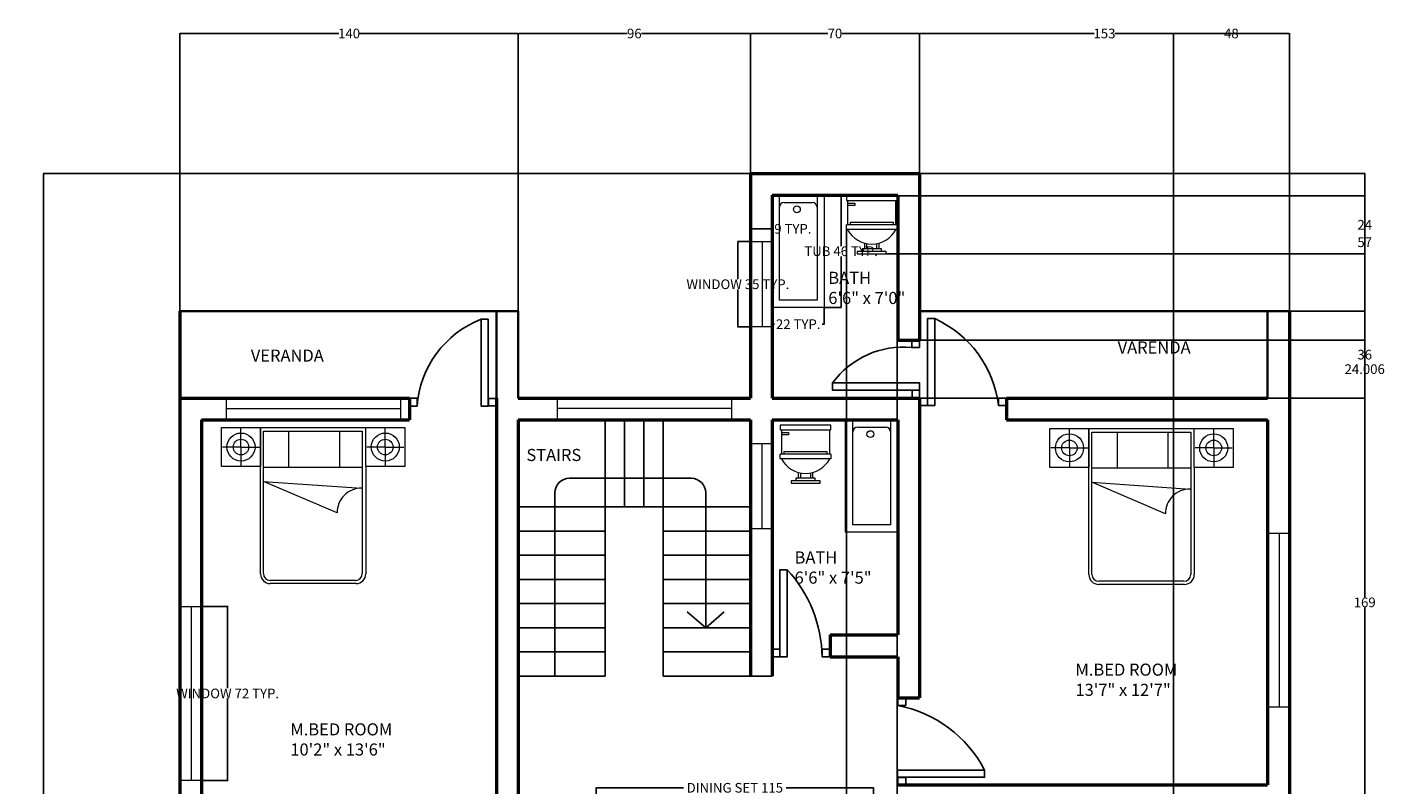
# Model space of a CAD drawing. Units: inches. Extents: x 870 to 1431, y 383 to 1070.
# Tile 9 of 9: x 870 to 1431, y 756 to 1070. Entities that reach past the tile are written whole.
import ezdxf

# ---------------------------------------------------------------- set-up
doc = ezdxf.new("R2010")
doc.units = ezdxf.units.IN
doc.header["$MEASUREMENT"] = 0
for name, color, linetype, lineweight in [('A-ANNO-DIMS', 2, 'Continuous', 18), ('A-AREA-IDEN', 7, 'Continuous', 25), ('A-DOOR', 3, 'Continuous', 25), ('A-FLOR-EXTR', 7, 'Continuous', 35), ('A-FLOR-FIXT', 9, 'Continuous', 18), ('A-FLOR-STRS', 7, 'Continuous', 25), ('A-FURN', 8, 'Continuous', 18), ('A-GLAZ', 4, 'Continuous', 18), ('A-WALL', 7, 'Continuous', 50)]:
    doc.layers.add(name, color=color, linetype=linetype, lineweight=lineweight)
doc.styles.get("Standard").update_dxf_attribs({"font": 'arial.ttf'})
doc.dimstyles.get("Standard").update_dxf_attribs({"dimtxt": 4, "dimasz": 0.18, "dimexe": 0.18, "dimexo": 0.0625, "dimgap": 0.09, "dimtad": 0, "dimtih": 1, "dimtoh": 1, "dimdec": 0, "dimrnd": 6, "dimzin": 0, "dimdsep": 46, "dimlunit": 3, "dimtxsty": 'Standard', "dimcen": 0.09, "dimadec": 0, "dimazin": 0, "dimtfac": 1, "dimtdec": 0, "dimtofl": 0, "dimtmove": 0, "dimatfit": 3, "dimfxl": 1, "dimtolj": 1, "dimtzin": 0, "dimarcsym": 0})

# ---------------------------------------------------------------- blocks, each defined once
blk = doc.blocks.new('A$C65997121')
for p, q in [((0, 1.5, -0.169), (0, 2, -0.169)), ((0, 2, -0.169), (0.5, 2, -0.169)), ((0, 1.5, -0.169), (0, 2, -0.169)), ((0, 2, -0.169), (0.5, 2, -0.169)), ((0.25, 1.75, -0.169), (0.25, 1.988, -0.169)), ((0.5, 2, -0.169), (1.755, 2, -0.169)), ((0.5, 2, -0.169), (1.512, 2, -0.169)), ((0.5, 2, -0.169), (1.512, 2, -0.169)), ((0.5, 0.125, -0.169), (0.5, 2, -0.169)), ((0.5, 2, -0.169), (0.5, 1.5, -0.169)), ((0.538, 1.488, -0.169), (0.538, 1.952, -0.169)), ((0.538, 1.952, -0.169), (1.805, 1.952, -0.169)), ((0.86, 1.952, -0.169), (0.86, 1.488, -0.169)), ((1.512, 2, -0.169), (2.35, 2, -0.169)), ((1.512, 2, -0.169), (2.35, 2, -0.169)), ((1.512, 1.952, -0.169), (1.512, 1.488, -0.169)), ((1.805, 1.952, -0.169), (1.805, 1.488, -0.169)), ((1.85, 2, -0.169), (2.35, 2, -0.169)), ((1.85, 1.5, -0.169), (1.85, 2, -0.169)), ((2.1, 1.75, -0.169), (2.1, 1.988, -0.169)), ((2.35, 2, -0.169), (2.35, 1.5, -0.169)), ((2.35, 2, -0.169), (2.35, 1.5, -0.169)), ((2.35, 2, -0.169), (2.35, 1.5, -0.169)), ((0.25, 1.75, -0.169), (0.012, 1.75, -0.169)), ((0.25, 1.75, -0.169), (0.25, 1.512, -0.169)), ((0.25, 1.75, -0.169), (0.488, 1.75, -0.169)), ((2.1, 1.75, -0.169), (1.862, 1.75, -0.169)), ((2.1, 1.75, -0.169), (2.338, 1.75, -0.169)), ((2.1, 1.75, -0.169), (2.1, 1.512, -0.169)), ((0.5, 1.5, -0.169), (0, 1.5, -0.169)), ((0.5, 1.5, -0.169), (0, 1.5, -0.169)), ((0.5, 0.125, -0.169), (0.5, 1.5, -0.169)), ((1.805, 1.488, -0.169), (0.538, 1.488, -0.169)), ((0.538, 0.128, -0.169), (0.538, 1.488, -0.169)), ((1.805, 1.488, -0.169), (1.805, 0.128, -0.169)), ((2.35, 1.5, -0.169), (1.85, 1.5, -0.169)), ((2.35, 1.5, -0.169), (1.85, 1.5, -0.169)), ((1.85, 1.5, -0.169), (1.85, 0.125, -0.169)), ((2.35, 1.5, -0.169), (1.85, 1.5, -0.169)), ((1.85, 1.5, -0.169), (1.85, 0.125, -0.169)), ((1.483, 0.905, -0.506), (0.538, 1.31, -0.506)), ((0.538, 1.31, -0.506), (1.797, 1.222, -0.506)), ((1.717, 0.04, -0.169), (0.625, 0.04, -0.169)), ((1.725, 0, -0.169), (0.625, 0, -0.169)), ((1.725, 0, -0.169), (0.625, 0, -0.169))]:
    blk.add_line(p, q)
for centre, radius in [((0.25, 1.75, -0.169), 0.18), ((2.1, 1.75, -0.169), 0.18), ((0.25, 1.75, -0.169), 0.1), ((2.1, 1.75, -0.169), 0.1)]:
    blk.add_circle(centre, radius)
for centre, radius, start, end in [((1.793, 0.911, -0.506), 0.311, 89.3268, 181.1229), ((0.625, 0.125, -0.169), 0.125, 179.9939, 269.9939), ((0.625, 0.125, -0.169), 0.125, 179.9939, 269.9939), ((0.625, 0.128, -0.169), 0.0875, 179.9939, 269.9939), ((1.717, 0.128, -0.169), 0.0875, 269.9939, 359.9939), ((1.725, 0.125, -0.169), 0.125, 269.9939, 359.9939), ((1.725, 0.125, -0.169), 0.125, 269.9939, 359.9939)]:
    blk.add_arc(centre, radius, start, end)
blk = doc.blocks.new('Toilet - Imperial')
for p, q in [((-10, 22), (-10, 12)), ((-10, 21), (-7, 21)), ((-7, 20), (-10, 20)), ((-7, 21), (-7, 20)), ((10, 12), (10, 22)), ((10.5, 12), (-10.5, 12)), ((-10.5, 10), (-10.5, 12)), ((9, 13), (-9, 13)), ((-9, 13), (-9, 12)), ((9, 12), (9, 13)), ((10.5, 12), (10.5, 10)), ((10.5, 10), (-10.5, 10)), ((4, 2), (-4, 2)), ((-4, 2), (-4, 1)), ((-3, 4.4065), (-3, 2)), ((-2, 2), (-2, 4.1658)), ((2, 4.1658), (2, 2)), ((3, 2), (3, 4.4065)), ((4, 1), (4, 2))]:
    blk.add_line(p, q)
for points in [[(10.5, 22), (10.5, 24), (-10.5, 24), (-10.5, 22)], [(6, 0), (6, 1), (-6, 1), (-6, 0)]]:
    blk.add_lwpolyline(points, close=True)
blk.add_arc((0, 15.3333), 11.3333, 208.0725, 331.9275)
blk = doc.blocks.new('WIN-72IN')
blk.add_line((4.72, 72), (4.72, 0))
blk.add_lwpolyline([(0, 72), (9, 72), (9, 0), (0, 0)], close=True)
blk = doc.blocks.new('WIN-BATH-35IN')
blk.add_line((4.73, 35.25), (4.73, 0))
blk.add_lwpolyline([(0, 0), (0, 35.25), (9, 35.25), (9, 0)], close=True)
blk = doc.blocks.new('BATH-TUB-COMPACT')
for p, q in [((0, 46.44), (21.59, 46.44)), ((0, 0), (0, 46.44)), ((3, 3), (3, 46.44)), ((18.59, 46.44), (18.59, 3)), ((21.59, 46.44), (21.59, 0)), ((5, 43.44), (16.59, 43.44)), ((21.59, 0), (0, 0)), ((18.59, 3), (3, 3))]:
    blk.add_line(p, q)
blk.add_circle((10.26, 40.55), 1.41)
for centre, start, end in [((5, 41.44), 90, 180), ((16.59, 41.44), 0, 90)]:
    blk.add_arc(centre, 2, start, end)
blk = doc.blocks.new('*D105')
at = {"layer": 'A-ANNO-DIMS', "color": 0, "lineweight": -2, "transparency": 16777216}
for p, q in [((941.8, 830.29), (952.72, 830.29)), ((952.54, 830.11), (952.54, 796.45)), ((952.54, 758.47), (952.54, 792.14)), ((941.8, 758.29), (952.72, 758.29))]:
    blk.add_line(p, q, dxfattribs=at)
at = {"layer": 'A-ANNO-DIMS', "color": 0, "transparency": 16777216}
for points in [[(952.51, 830.11), (952.57, 830.11), (952.54, 830.29)], [(952.51, 758.47), (952.57, 758.47), (952.54, 758.29)]]:
    blk.add_solid(points, dxfattribs=at)
at = {"layer": 'Defpoints', "color": 0, "transparency": 16777216}
for p in [(941.74, 830.29), (952.54, 830.29), (941.74, 758.29)]:
    blk.add_point(p, dxfattribs=at)
at = {"layer": 'A-ANNO-DIMS', "color": 0, "transparency": 16777216, "insert": (952.54, 794.29), "char_height": 4, "attachment_point": 5}
blk.add_mtext('\\A1;WINDOW 72 TYP.', dxfattribs=at)
blk = doc.blocks.new('*D106')
at = {"layer": 'A-ANNO-DIMS', "color": 0, "lineweight": -2, "transparency": 16777216}
for p, q in [((932.74, 758.23), (932.74, 747.31)), ((941.74, 758.23), (941.74, 747.31)), ((932.92, 747.49), (941.56, 747.49)), ((941.74, 747.49), (941.92, 747.49))]:
    blk.add_line(p, q, dxfattribs=at)
at = {"layer": 'A-ANNO-DIMS', "color": 0, "transparency": 16777216}
for points in [[(932.92, 747.52), (932.92, 747.46), (932.74, 747.49)], [(941.56, 747.52), (941.56, 747.46), (941.74, 747.49)]]:
    blk.add_solid(points, dxfattribs=at)
at = {"layer": 'Defpoints', "color": 0, "transparency": 16777216}
for p in [(932.74, 758.29), (941.74, 758.29), (941.74, 747.49)]:
    blk.add_point(p, dxfattribs=at)
at = {"layer": 'A-ANNO-DIMS', "color": 0, "transparency": 16777216, "insert": (950.19, 747.49), "char_height": 4, "attachment_point": 5}
blk.add_mtext('\\A1;9 TYP.', dxfattribs=at)
blk = doc.blocks.new('*D111')
at = {"layer": 'A-ANNO-DIMS', "color": 0, "lineweight": -2, "transparency": 16777216}
for p, q in [((1168.86, 981.23), (1163.46, 981.23)), ((1163.64, 981.05), (1163.64, 965.76)), ((1163.64, 946.16), (1163.64, 961.44)), ((1168.86, 945.98), (1163.46, 945.98))]:
    blk.add_line(p, q, dxfattribs=at)
at = {"layer": 'A-ANNO-DIMS', "color": 0, "transparency": 16777216}
for points in [[(1163.61, 981.05), (1163.67, 981.05), (1163.64, 981.23)], [(1163.61, 946.16), (1163.67, 946.16), (1163.64, 945.98)]]:
    blk.add_solid(points, dxfattribs=at)
at = {"layer": 'Defpoints', "color": 0, "transparency": 16777216}
for p in [(1163.64, 981.23), (1168.93, 981.23), (1168.93, 945.98)]:
    blk.add_point(p, dxfattribs=at)
at = {"layer": 'A-ANNO-DIMS', "color": 0, "transparency": 16777216, "insert": (1163.64, 963.6), "char_height": 4, "attachment_point": 5}
blk.add_mtext('\\A1;WINDOW 35 TYP.', dxfattribs=at)
blk = doc.blocks.new('*D112')
at = {"layer": 'A-ANNO-DIMS', "color": 0, "lineweight": -2, "transparency": 16777216}
for p, q in [((1168.93, 981.29), (1168.93, 986.7)), ((1169.11, 986.52), (1177.75, 986.52)), ((1177.93, 981.29), (1177.93, 986.7)), ((1177.93, 986.52), (1178.11, 986.52))]:
    blk.add_line(p, q, dxfattribs=at)
at = {"layer": 'A-ANNO-DIMS', "color": 0, "transparency": 16777216}
for points in [[(1169.11, 986.55), (1169.11, 986.49), (1168.93, 986.52)], [(1177.75, 986.55), (1177.75, 986.49), (1177.93, 986.52)]]:
    blk.add_solid(points, dxfattribs=at)
at = {"layer": 'Defpoints', "color": 0, "transparency": 16777216}
for p in [(1177.93, 986.52), (1168.93, 981.23), (1177.93, 981.23)]:
    blk.add_point(p, dxfattribs=at)
at = {"layer": 'A-ANNO-DIMS', "color": 0, "transparency": 16777216, "insert": (1186.38, 986.52), "char_height": 4, "attachment_point": 5}
blk.add_mtext('\\A1;9 TYP.', dxfattribs=at)
blk = doc.blocks.new('*D119')
at = {"layer": 'A-ANNO-DIMS', "color": 0, "lineweight": -2, "transparency": 16777216}
for p, q in [((1199.45, 1000.48), (1206.53, 1000.48)), ((1206.35, 1000.3), (1206.35, 979.39)), ((1206.35, 954.22), (1206.35, 975.13)), ((1199.45, 954.04), (1206.53, 954.04))]:
    blk.add_line(p, q, dxfattribs=at)
at = {"layer": 'A-ANNO-DIMS', "color": 0, "transparency": 16777216}
for points in [[(1206.32, 1000.3), (1206.38, 1000.3), (1206.35, 1000.48)], [(1206.32, 954.22), (1206.38, 954.22), (1206.35, 954.04)]]:
    blk.add_solid(points, dxfattribs=at)
at = {"layer": 'Defpoints', "color": 0, "transparency": 16777216}
for p in [(1199.38, 1000.48), (1206.35, 1000.48), (1199.38, 954.04)]:
    blk.add_point(p, dxfattribs=at)
at = {"layer": 'A-ANNO-DIMS', "color": 0, "transparency": 16777216, "insert": (1206.35, 977.26), "char_height": 4, "attachment_point": 5}
blk.add_mtext('\\A1;TUB 46 TYP.', dxfattribs=at)
blk = doc.blocks.new('*D120')
at = {"layer": 'A-ANNO-DIMS', "color": 0, "lineweight": -2, "transparency": 16777216}
for p, q in [((1177.79, 953.98), (1177.79, 946.89)), ((1199.38, 953.98), (1199.38, 946.89)), ((1177.97, 947.07), (1178.73, 947.07)), ((1199.2, 947.07), (1198.45, 947.07))]:
    blk.add_line(p, q, dxfattribs=at)
at = {"layer": 'A-ANNO-DIMS', "color": 0, "transparency": 16777216}
for points in [[(1177.97, 947.1), (1177.97, 947.04), (1177.79, 947.07)], [(1199.2, 947.1), (1199.2, 947.04), (1199.38, 947.07)]]:
    blk.add_solid(points, dxfattribs=at)
at = {"layer": 'Defpoints', "color": 0, "transparency": 16777216}
for p in [(1177.79, 954.04), (1199.38, 954.04), (1199.38, 947.07)]:
    blk.add_point(p, dxfattribs=at)
at = {"layer": 'A-ANNO-DIMS', "color": 0, "transparency": 16777216, "insert": (1188.59, 947.07), "char_height": 4, "attachment_point": 5}
blk.add_mtext('\\A1;22 TYP.', dxfattribs=at)
blk = doc.blocks.new('*D123')
at = {"layer": 'A-ANNO-DIMS', "color": 0, "lineweight": -2, "transparency": 16777216}
for p, q in [((1104.97, 738.1), (1104.97, 755.44)), ((1105.15, 755.26), (1141.18, 755.26)), ((1219.6, 755.26), (1183.56, 755.26)), ((1219.78, 738.1), (1219.78, 755.44))]:
    blk.add_line(p, q, dxfattribs=at)
at = {"layer": 'A-ANNO-DIMS', "color": 0, "transparency": 16777216}
for points in [[(1105.15, 755.29), (1105.15, 755.23), (1104.97, 755.26)], [(1219.6, 755.29), (1219.6, 755.23), (1219.78, 755.26)]]:
    blk.add_solid(points, dxfattribs=at)
at = {"layer": 'Defpoints', "color": 0, "transparency": 16777216}
for p in [(1219.78, 755.26), (1104.97, 738.04), (1219.78, 738.04)]:
    blk.add_point(p, dxfattribs=at)
at = {"layer": 'A-ANNO-DIMS', "color": 0, "transparency": 16777216, "insert": (1162.37, 755.26), "char_height": 4, "attachment_point": 5}
blk.add_mtext('\\A1;DINING SET 115', dxfattribs=at)
blk = doc.blocks.new('*D126')
at = {"layer": 'A-ANNO-DIMS', "color": 0, "lineweight": -2, "transparency": 16777216}
for p, q in [((1168.73, 1009.48), (876.24, 1009.48)), ((876.42, 1009.3), (876.42, 715.17)), ((876.42, 416.77), (876.42, 710.9)), ((1094.63, 416.59), (876.24, 416.59))]:
    blk.add_line(p, q, dxfattribs=at)
at = {"layer": 'A-ANNO-DIMS', "color": 0, "transparency": 16777216}
for points in [[(876.39, 1009.3), (876.45, 1009.3), (876.42, 1009.48)], [(876.39, 416.77), (876.45, 416.77), (876.42, 416.59)]]:
    blk.add_solid(points, dxfattribs=at)
at = {"layer": 'Defpoints', "color": 0, "transparency": 16777216}
for p in [(876.42, 1009.48), (1168.79, 1009.48), (1094.7, 416.59)]:
    blk.add_point(p, dxfattribs=at)
at = {"layer": 'A-ANNO-DIMS', "color": 0, "transparency": 16777216, "insert": (876.42, 713.03), "char_height": 4, "attachment_point": 5}
blk.add_mtext('\\A1;592.9', dxfattribs=at)
blk = doc.blocks.new('*D127')
at = {"layer": 'A-ANNO-DIMS', "color": 0, "lineweight": -2, "transparency": 16777216}
for p, q in [((932.79, 952.54), (932.79, 1067.52)), ((932.97, 1067.34), (998.48, 1067.34)), ((1072.61, 1067.34), (1007.1, 1067.34)), ((1072.79, 952.54), (1072.79, 1067.52))]:
    blk.add_line(p, q, dxfattribs=at)
at = {"layer": 'A-ANNO-DIMS', "color": 0, "transparency": 16777216}
for points in [[(932.97, 1067.37), (932.97, 1067.31), (932.79, 1067.34)], [(1072.61, 1067.37), (1072.61, 1067.31), (1072.79, 1067.34)]]:
    blk.add_solid(points, dxfattribs=at)
at = {"layer": 'Defpoints', "color": 0, "transparency": 16777216}
for p in [(1072.79, 1067.34), (932.79, 952.48), (1072.79, 952.48)]:
    blk.add_point(p, dxfattribs=at)
at = {"layer": 'A-ANNO-DIMS', "color": 0, "transparency": 16777216, "insert": (1002.79, 1067.34), "char_height": 4, "attachment_point": 5}
blk.add_mtext('\\A1;140', dxfattribs=at)
blk = doc.blocks.new('*D128')
at = {"layer": 'A-ANNO-DIMS', "color": 0, "lineweight": -2, "transparency": 16777216}
for p, q in [((1072.79, 952.54), (1072.79, 1067.52)), ((1072.97, 1067.34), (1117.84, 1067.34)), ((1168.61, 1067.34), (1123.74, 1067.34)), ((1168.79, 916.54), (1168.79, 1067.52))]:
    blk.add_line(p, q, dxfattribs=at)
at = {"layer": 'A-ANNO-DIMS', "color": 0, "transparency": 16777216}
for points in [[(1072.97, 1067.37), (1072.97, 1067.31), (1072.79, 1067.34)], [(1168.61, 1067.37), (1168.61, 1067.31), (1168.79, 1067.34)]]:
    blk.add_solid(points, dxfattribs=at)
at = {"layer": 'Defpoints', "color": 0, "transparency": 16777216}
for p in [(1168.79, 1067.34), (1072.79, 952.48), (1168.79, 916.48)]:
    blk.add_point(p, dxfattribs=at)
at = {"layer": 'A-ANNO-DIMS', "color": 0, "transparency": 16777216, "insert": (1120.79, 1067.34), "char_height": 4, "attachment_point": 5}
blk.add_mtext('\\A1;96', dxfattribs=at)
blk = doc.blocks.new('*D129')
at = {"layer": 'A-ANNO-DIMS', "color": 0, "lineweight": -2, "transparency": 16777216}
for p, q in [((1168.79, 1009.54), (1168.79, 1067.52)), ((1168.97, 1067.34), (1200.86, 1067.34)), ((1238.61, 1067.34), (1206.72, 1067.34)), ((1238.79, 1009.54), (1238.79, 1067.52))]:
    blk.add_line(p, q, dxfattribs=at)
at = {"layer": 'A-ANNO-DIMS', "color": 0, "transparency": 16777216}
for points in [[(1168.97, 1067.37), (1168.97, 1067.31), (1168.79, 1067.34)], [(1238.61, 1067.37), (1238.61, 1067.31), (1238.79, 1067.34)]]:
    blk.add_solid(points, dxfattribs=at)
at = {"layer": 'Defpoints', "color": 0, "transparency": 16777216}
for p in [(1238.79, 1067.34), (1168.79, 1009.48), (1238.79, 1009.48)]:
    blk.add_point(p, dxfattribs=at)
at = {"layer": 'A-ANNO-DIMS', "color": 0, "transparency": 16777216, "insert": (1203.79, 1067.34), "char_height": 4, "attachment_point": 5}
blk.add_mtext('\\A1;70', dxfattribs=at)
blk = doc.blocks.new('*D130')
at = {"layer": 'A-ANNO-DIMS', "color": 0, "lineweight": -2, "transparency": 16777216}
for p, q in [((1238.79, 952.54), (1238.79, 1067.52)), ((1238.97, 1067.34), (1310.97, 1067.34)), ((1391.61, 1067.34), (1319.61, 1067.34)), ((1391.79, 952.54), (1391.79, 1067.52))]:
    blk.add_line(p, q, dxfattribs=at)
at = {"layer": 'A-ANNO-DIMS', "color": 0, "transparency": 16777216}
for points in [[(1238.97, 1067.37), (1238.97, 1067.31), (1238.79, 1067.34)], [(1391.61, 1067.37), (1391.61, 1067.31), (1391.79, 1067.34)]]:
    blk.add_solid(points, dxfattribs=at)
at = {"layer": 'Defpoints', "color": 0, "transparency": 16777216}
for p in [(1391.79, 1067.34), (1238.79, 952.48), (1391.79, 952.48)]:
    blk.add_point(p, dxfattribs=at)
at = {"layer": 'A-ANNO-DIMS', "color": 0, "transparency": 16777216, "insert": (1315.29, 1067.34), "char_height": 4, "attachment_point": 5}
blk.add_mtext('\\A1;153', dxfattribs=at)
blk = doc.blocks.new('*D131')
at = {"layer": 'A-ANNO-DIMS', "color": 0, "lineweight": -2, "transparency": 16777216}
for p, q in [((1238.85, 1009.48), (1423.14, 1009.48)), ((1422.96, 1009.3), (1422.96, 983.1)), ((1422.96, 952.66), (1422.96, 978.85)), ((1391.85, 952.48), (1423.14, 952.48))]:
    blk.add_line(p, q, dxfattribs=at)
at = {"layer": 'A-ANNO-DIMS', "color": 0, "transparency": 16777216}
for points in [[(1422.93, 1009.3), (1422.99, 1009.3), (1422.96, 1009.48)], [(1422.93, 952.66), (1422.99, 952.66), (1422.96, 952.48)]]:
    blk.add_solid(points, dxfattribs=at)
at = {"layer": 'Defpoints', "color": 0, "transparency": 16777216}
for p in [(1238.79, 1009.48), (1391.79, 952.48), (1422.96, 952.48)]:
    blk.add_point(p, dxfattribs=at)
at = {"layer": 'A-ANNO-DIMS', "color": 0, "transparency": 16777216, "insert": (1422.96, 980.98), "char_height": 4, "attachment_point": 5}
blk.add_mtext('\\A1;57', dxfattribs=at)
blk = doc.blocks.new('*D132')
at = {"layer": 'A-ANNO-DIMS', "color": 0, "lineweight": -2, "transparency": 16777216}
for p, q in [((1391.85, 952.48), (1423.14, 952.48)), ((1422.96, 952.3), (1422.96, 936.61)), ((1422.96, 916.66), (1422.96, 932.34)), ((1382.85, 916.48), (1423.14, 916.48))]:
    blk.add_line(p, q, dxfattribs=at)
at = {"layer": 'A-ANNO-DIMS', "color": 0, "transparency": 16777216}
for points in [[(1422.93, 952.3), (1422.99, 952.3), (1422.96, 952.48)], [(1422.93, 916.66), (1422.99, 916.66), (1422.96, 916.48)]]:
    blk.add_solid(points, dxfattribs=at)
at = {"layer": 'Defpoints', "color": 0, "transparency": 16777216}
for p in [(1391.79, 952.48), (1382.79, 916.48), (1422.96, 916.48)]:
    blk.add_point(p, dxfattribs=at)
at = {"layer": 'A-ANNO-DIMS', "color": 0, "transparency": 16777216, "insert": (1422.96, 934.48), "char_height": 4, "attachment_point": 5}
blk.add_mtext('\\A1;36', dxfattribs=at)
blk = doc.blocks.new('*D133')
at = {"layer": 'A-ANNO-DIMS', "color": 0, "lineweight": -2, "transparency": 16777216}
for p, q in [((1382.85, 916.48), (1423.14, 916.48)), ((1422.96, 916.3), (1422.96, 834.11)), ((1422.96, 747.66), (1422.96, 829.84)), ((1391.85, 747.48), (1423.14, 747.48))]:
    blk.add_line(p, q, dxfattribs=at)
at = {"layer": 'A-ANNO-DIMS', "color": 0, "transparency": 16777216}
for points in [[(1422.93, 916.3), (1422.99, 916.3), (1422.96, 916.48)], [(1422.93, 747.66), (1422.99, 747.66), (1422.96, 747.48)]]:
    blk.add_solid(points, dxfattribs=at)
at = {"layer": 'Defpoints', "color": 0, "transparency": 16777216}
for p in [(1382.79, 916.48), (1391.79, 747.48), (1422.96, 747.48)]:
    blk.add_point(p, dxfattribs=at)
at = {"layer": 'A-ANNO-DIMS', "color": 0, "transparency": 16777216, "insert": (1422.96, 831.98), "char_height": 4, "attachment_point": 5}
blk.add_mtext('\\A1;169', dxfattribs=at)
blk = doc.blocks.new('*D136')
at = {"layer": 'A-ANNO-DIMS', "color": 0, "lineweight": -2, "transparency": 16777216}
for p, q in [((1208.53, 986.13), (1208.53, 385.26)), ((1229.53, 986.13), (1229.53, 385.26)), ((1208.71, 385.44), (1216.43, 385.44)), ((1229.35, 385.44), (1221.64, 385.44))]:
    blk.add_line(p, q, dxfattribs=at)
at = {"layer": 'A-ANNO-DIMS', "color": 0, "transparency": 16777216}
for points in [[(1208.71, 385.47), (1208.71, 385.41), (1208.53, 385.44)], [(1229.35, 385.47), (1229.35, 385.41), (1229.53, 385.44)]]:
    blk.add_solid(points, dxfattribs=at)
at = {"layer": 'Defpoints', "color": 0, "transparency": 16777216}
for p in [(1208.53, 986.19), (1229.53, 986.19), (1229.53, 385.44)]:
    blk.add_point(p, dxfattribs=at)
at = {"layer": 'A-ANNO-DIMS', "color": 0, "transparency": 16777216, "insert": (1219.03, 385.44), "char_height": 4, "attachment_point": 5}
blk.add_mtext('\\A1;21', dxfattribs=at)
blk = doc.blocks.new('*D137')
at = {"layer": 'A-ANNO-DIMS', "color": 0, "lineweight": -2, "transparency": 16777216}
for p, q in [((1229.6, 1000.19), (1423.14, 1000.19)), ((1422.96, 1000.01), (1422.96, 990.29)), ((1422.96, 976.37), (1422.96, 986.09)), ((1225.1, 976.19), (1423.14, 976.19))]:
    blk.add_line(p, q, dxfattribs=at)
at = {"layer": 'A-ANNO-DIMS', "color": 0, "transparency": 16777216}
for points in [[(1422.93, 1000.01), (1422.99, 1000.01), (1422.96, 1000.19)], [(1422.93, 976.37), (1422.99, 976.37), (1422.96, 976.19)]]:
    blk.add_solid(points, dxfattribs=at)
at = {"layer": 'Defpoints', "color": 0, "transparency": 16777216}
for p in [(1229.53, 1000.19), (1225.03, 976.19), (1422.96, 976.19)]:
    blk.add_point(p, dxfattribs=at)
at = {"layer": 'A-ANNO-DIMS', "color": 0, "transparency": 16777216, "insert": (1422.96, 988.19), "char_height": 4, "attachment_point": 5}
blk.add_mtext('\\A1;24', dxfattribs=at)
blk = doc.blocks.new('*D138')
at = {"layer": 'A-ANNO-DIMS', "color": 0, "lineweight": -2, "transparency": 16777216}
for p, q in [((1343.79, 640.54), (1343.79, 1067.52)), ((1343.97, 1067.34), (1364.75, 1067.34)), ((1391.61, 1067.34), (1370.83, 1067.34)), ((1391.79, 640.54), (1391.79, 1067.52))]:
    blk.add_line(p, q, dxfattribs=at)
at = {"layer": 'A-ANNO-DIMS', "color": 0, "transparency": 16777216}
for points in [[(1343.97, 1067.37), (1343.97, 1067.31), (1343.79, 1067.34)], [(1391.61, 1067.37), (1391.61, 1067.31), (1391.79, 1067.34)]]:
    blk.add_solid(points, dxfattribs=at)
at = {"layer": 'Defpoints', "color": 0, "transparency": 16777216}
for p in [(1391.79, 1067.34), (1343.79, 640.48), (1391.79, 640.48)]:
    blk.add_point(p, dxfattribs=at)
at = {"layer": 'A-ANNO-DIMS', "color": 0, "transparency": 16777216, "insert": (1367.79, 1067.34), "char_height": 4, "attachment_point": 5}
blk.add_mtext('\\A1;48', dxfattribs=at)
blk = doc.blocks.new('*D142')
at = {"layer": 'A-ANNO-DIMS', "color": 0, "lineweight": -2, "transparency": 16777216}
for p, q in [((1238.89, 940.48), (1423.14, 940.48)), ((1422.96, 940.3), (1422.96, 930.61)), ((1422.96, 916.66), (1422.96, 926.35)), ((1238.85, 916.48), (1423.14, 916.48))]:
    blk.add_line(p, q, dxfattribs=at)
at = {"layer": 'A-ANNO-DIMS', "color": 0, "transparency": 16777216}
for points in [[(1422.93, 940.3), (1422.99, 940.3), (1422.96, 940.48)], [(1422.93, 916.66), (1422.99, 916.66), (1422.96, 916.48)]]:
    blk.add_solid(points, dxfattribs=at)
at = {"layer": 'Defpoints', "color": 0, "transparency": 16777216}
for p in [(1238.83, 940.48), (1422.96, 940.48), (1238.79, 916.48)]:
    blk.add_point(p, dxfattribs=at)
at = {"layer": 'A-ANNO-DIMS', "color": 0, "transparency": 16777216, "insert": (1422.96, 928.48), "char_height": 4, "attachment_point": 5}
blk.add_mtext('\\A1;24.006', dxfattribs=at)

msp = doc.modelspace()

# ---------------------------------------------------------------- linework, layer by layer
at = {"layer": 'A-DOOR'}
for points in [[(1245.0601, 949.3759), (1245.0601, 913.3759), (1242.0601, 913.3759), (1242.0601, 949.3759)], [(1060.392, 949.1701), (1060.392, 913.1701), (1057.392, 913.1701), (1057.392, 949.1701)], [(1238.8258, 937.3818), (1235.5564, 937.3818), (1235.5564, 940.4832), (1238.8258, 940.4832)], [(1202.7907, 922.7466), (1238.7907, 922.7466), (1238.7907, 919.7466), (1202.7907, 919.7466)], [(1027.7907, 913.2078), (1027.7907, 916.4772), (1030.8921, 916.4772), (1030.8921, 913.2078)], [(1063.7316, 913.2642), (1060.4623, 913.2642), (1060.4623, 916.3655), (1063.7316, 916.3655)], [(1238.7907, 919.7466), (1238.7907, 916.4772), (1235.6894, 916.4772), (1235.6894, 919.7466)], [(1238.7907, 919.7466), (1238.7907, 916.4772), (1235.6894, 916.4772), (1235.6894, 919.7466)], [(1242.0601, 913.3759), (1238.7907, 913.3759), (1238.7907, 916.4772), (1242.0601, 916.4772)], [(1274.7907, 913.3771), (1271.5214, 913.3771), (1271.5214, 916.4785), (1274.7907, 916.4785)], [(1184.0601, 845.4772), (1184.0601, 809.4772), (1181.0601, 809.4772), (1181.0601, 845.4772)], [(1181.0601, 809.4772), (1177.7907, 809.4772), (1177.7907, 812.5786), (1181.0601, 812.5786)], [(1201.7871, 809.474), (1198.5177, 809.474), (1198.5177, 812.5753), (1201.7871, 812.5753)], [(1233.0667, 789.3158), (1229.7973, 789.3158), (1229.7973, 792.4171), (1233.0667, 792.4171)], [(1229.7226, 762.5985), (1265.7226, 762.5985), (1265.7226, 759.5985), (1229.7226, 759.5985)], [(1233.0601, 756.4772), (1229.7907, 756.4772), (1229.7907, 759.5786), (1233.0601, 759.5786)]]:
    msp.add_lwpolyline(points, close=True, dxfattribs=at)
for centre, radius, start, end in [((1226.0518, 907.6789), 45.8253, 7.14304, 65.493232), ((1072.9308, 909.9751), 42.1628, 111.625713, 175.60261), ((1231.9812, 901.3903), 36.1687, 84.327182, 143.810072), ((1143.9677, 808.4731), 54.5592, 1.051159, 42.706121), ((1220.0694, 738.723), 51.5195, 27.608473, 79.11601)]:
    msp.add_arc(centre, radius, start, end, dxfattribs=at)
at = {"layer": 'A-FLOR-EXTR'}
for p, q in [((932.7907, 952.4772), (1072.7907, 952.4772)), ((1063.7907, 952.4772), (1063.7907, 916.4772)), ((1072.7907, 952.4772), (1072.7907, 916.4772)), ((1238.7907, 952.4772), (1391.7907, 952.4772)), ((1382.7907, 952.4772), (1382.7907, 916.4772))]:
    msp.add_line(p, q, dxfattribs=at)
at = {"layer": 'A-FLOR-STRS'}
for p, q in [((1108.7907, 907.4772), (1108.7907, 801.4772)), ((1116.7907, 907.4772), (1116.7907, 871.4772)), ((1124.7907, 907.4772), (1124.7907, 871.4772)), ((1132.7907, 907.4772), (1132.7907, 801.4772)), ((1093.9228, 883.3419), (1144.3123, 883.3419)), ((1087.9228, 801.4772), (1087.9228, 877.3419)), ((1150.3123, 877.3419), (1150.3123, 821.4772)), ((1072.7907, 871.4772), (1168.7907, 871.4772)), ((1072.7907, 861.4772), (1108.7907, 861.4772)), ((1132.7907, 861.4772), (1168.7907, 861.4772)), ((1072.7907, 851.4772), (1108.7907, 851.4772)), ((1132.7907, 851.4772), (1168.7907, 851.4772)), ((1072.7907, 841.4772), (1108.7907, 841.4772)), ((1132.7907, 841.4772), (1168.7907, 841.4772)), ((1072.7907, 831.4772), (1108.7907, 831.4772)), ((1132.7907, 831.4772), (1168.7907, 831.4772)), ((1150.3123, 821.4772), (1142.7145, 828.0448)), ((1150.3123, 821.4772), (1157.9102, 828.0448)), ((1072.7907, 821.4772), (1108.7907, 821.4772)), ((1132.7907, 821.4772), (1168.7907, 821.4772)), ((1072.7907, 811.4772), (1108.7907, 811.4772)), ((1132.7907, 811.4772), (1168.7907, 811.4772)), ((1072.7907, 801.4772), (1108.7907, 801.4772)), ((1132.7907, 801.4772), (1177.7907, 801.4772))]:
    msp.add_line(p, q, dxfattribs=at)
for centre, start, end in [((1093.9228, 877.3419), 90, 180), ((1144.3123, 877.3419), 0, 90)]:
    msp.add_arc(centre, 6, start, end, dxfattribs=at)
at = {"layer": 'A-WALL'}
for p, q in [((1168.7907, 1009.4772), (1168.7907, 916.4772)), ((1168.7907, 1009.4772), (1238.7907, 1009.4772)), ((1238.7907, 1009.4772), (1238.7907, 940.4772)), ((1177.7907, 1000.4772), (1177.7907, 916.4772)), ((1177.7907, 1000.4772), (1229.7907, 1000.4772)), ((1229.7907, 1000.4772), (1229.7907, 940.4772)), ((932.7907, 952.4772), (932.7907, 427.4772)), ((1391.7907, 952.4772), (1391.7907, 747.4772)), ((1229.7907, 940.4772), (1238.7907, 940.4772)), ((932.7907, 916.4772), (1027.7907, 916.4772)), ((1027.7907, 916.4772), (1027.7907, 907.4772)), ((1063.7907, 916.4772), (1063.7907, 734.4772)), ((1072.7907, 916.4772), (1168.7907, 916.4772)), ((1177.7907, 916.4772), (1229.7907, 916.4772)), ((1229.7907, 916.4772), (1238.7907, 916.4772)), ((1238.7907, 916.4772), (1238.7907, 792.4772)), ((1274.7907, 916.4772), (1274.7907, 907.4772)), ((1274.7907, 916.4772), (1382.7907, 916.4772)), ((941.7907, 907.4772), (1027.7907, 907.4772)), ((941.7907, 907.4772), (941.7907, 510.4772)), ((1072.7907, 907.4772), (1072.7907, 734.4772)), ((1072.7907, 907.4772), (1168.7907, 907.4772)), ((1168.7907, 907.4772), (1168.7907, 801.4772)), ((1177.7907, 907.4772), (1177.7907, 809.4772)), ((1177.7907, 907.4772), (1229.7907, 907.4772)), ((1229.7907, 907.4772), (1229.7907, 818.4772)), ((1274.7907, 907.4772), (1382.7907, 907.4772)), ((1382.7907, 907.4772), (1382.7907, 756.4772)), ((1201.7907, 818.4772), (1229.7907, 818.4772)), ((1201.7907, 818.4772), (1201.7907, 809.4772)), ((1177.7907, 809.4772), (1177.7907, 801.4772)), ((1201.7907, 809.4772), (1229.7907, 809.4772)), ((1229.7907, 809.4772), (1229.7907, 792.4772)), ((1229.7907, 809.4772), (1229.7907, 792.4772)), ((1229.7907, 792.4772), (1238.7907, 792.4772)), ((1229.7907, 756.4772), (1382.7907, 756.4772))]:
    msp.add_line(p, q, dxfattribs=at)

# ---------------------------------------------------------------- block references
at = {"layer": 'A-FLOR-FIXT'}
for name, p in [('BATH-TUB-COMPACT', (1177.791, 954.04)), ('Toilet - Imperial', (1219.0328, 976.1907)), ('Toilet - Imperial', (1191.6184, 881.3119)), ('BATH-TUB-COMPACT', (1208.1981, 861.04))]:
    msp.add_blockref(name, p, dxfattribs=at)
at = {"layer": 'A-FURN', "xscale": 32.26790700275002, "yscale": 32.26790700275002, "zscale": 32.26790700275002}
for p in [(950.005, 839.7696, 5.4452), (1292.7289, 839.4244, 5.4452)]:
    msp.add_blockref('A$C65997121', p, dxfattribs=at)
at = {"layer": 'A-GLAZ'}
for name, p in [('WIN-BATH-35IN', (1168.9261, 945.9755)), ('WIN-BATH-35IN', (1168.861, 862.4422)), ('WIN-72IN', (1382.8083, 788.5788)), ('WIN-72IN', (932.7364, 758.2945))]:
    msp.add_blockref(name, p, dxfattribs=at)
for p, rotation in [((1024.102, 907.4029), 89.99999999999969), ((1160.9883, 907.6037), 89.99999999999972)]:
    msp.add_blockref('WIN-72IN', p, dxfattribs=dict(at, rotation=rotation))

# ---------------------------------------------------------------- texts
at = {"layer": 'A-AREA-IDEN', "char_height": 5, "attachment_point": 1}
for s, insert in [('BATH\\P6\'6" x 7\'0"', (1201.0496, 968.7493)), ('VARENDA', (1320.7503, 939.9355)), ('VERANDA', (962.1404, 936.583)), ('STAIRS', (1076.1532, 895.4544)), ('BATH\\P6\'6" x 7\'5"', (1187.0837, 853.0461)), ('M.BED ROOM\\P13\'7" x 12\'7"', (1303.2888, 806.6381)), ('M.BED ROOM\\P10\'2" x 13\'6"', (978.489, 781.9319))]:
    msp.add_mtext_dynamic_manual_height_columns(s, width=69.132678, gutter_width=1, heights=[0], dxfattribs=dict(at, insert=insert))

# ---------------------------------------------------------------- dimensions: what is measured, and where the dimension line sits
at = {"layer": 'A-ANNO-DIMS'}
for base, p1, p2, picture, middle in [((1072.7907, 1067.3407), (932.7907, 952.4772), (1072.7907, 952.4772), '*D127', (1002.7907, 1067.3407)), ((1168.7907, 1067.3407), (1072.7907, 952.4772), (1168.7907, 916.4772), '*D128', (1120.7907, 1067.3407)), ((1238.7907, 1067.3407), (1168.7907, 1009.4772), (1238.7907, 1009.4772), '*D129', (1203.7907, 1067.3407)), ((1391.7907, 1067.3407), (1238.7907, 952.4772), (1391.7907, 952.4772), '*D130', (1315.2907, 1067.3407)), ((1391.7907, 1067.3407), (1343.7907, 640.4772), (1391.7907, 640.4772), '*D138', (1367.7907, 1067.3407)), ((1229.5328, 385.44), (1208.5328, 986.1907), (1229.5328, 986.1907), '*D136', (1219.0328, 385.44))]:
    dim = msp.add_linear_dim(base=base, p1=p1, p2=p2, dimstyle='Standard', override={"dimdec": 0, "dimlfac": 1, "dimrnd": 0, "dimzin": 0, "dimdsep": 46, "dimlunit": 2}, dxfattribs=at)
    dim.commit()
    dim.dimension.update_dxf_attribs({"geometry": picture, "text_midpoint": middle})
for base, p1, p2, override, picture, middle in [((876.4215, 1009.4772), (1094.6967, 416.59), (1168.7907, 1009.4772), {"dimdec": 1, "dimlfac": 1, "dimrnd": 0, "dimzin": 0, "dimdsep": 46, "dimlunit": 2}, '*D126', (876.4215, 713.0336)), ((1422.9581, 952.4772), (1238.7907, 1009.4772), (1391.7907, 952.4772), {"dimdec": 0, "dimlfac": 1, "dimrnd": 0, "dimzin": 0, "dimdsep": 46, "dimlunit": 2}, '*D131', (1422.9581, 980.9772)), ((1422.9581, 976.1907), (1229.5328, 1000.1907), (1225.0328, 976.1907), {"dimdec": 0, "dimlfac": 1, "dimrnd": 0, "dimzin": 0, "dimdsep": 46, "dimlunit": 2}, '*D137', (1422.9581, 988.1907)), ((1422.9581, 916.4772), (1391.7907, 952.4772), (1382.7907, 916.4772), {"dimdec": 0, "dimlfac": 1, "dimrnd": 0, "dimzin": 0, "dimdsep": 46, "dimlunit": 2}, '*D132', (1422.9581, 934.4772)), ((1422.9581, 940.4832), (1238.7907, 916.4772), (1238.8258, 940.4832), {"dimdec": 3, "dimlfac": 1, "dimrnd": 0, "dimzin": 0, "dimdsep": 46, "dimlunit": 2}, '*D142', (1422.9581, 928.4802)), ((1422.9581, 747.4772), (1382.7907, 916.4772), (1391.7907, 747.4772), {"dimdec": 0, "dimlfac": 1, "dimrnd": 0, "dimzin": 0, "dimdsep": 46, "dimlunit": 2}, '*D133', (1422.9581, 831.9772))]:
    dim = msp.add_linear_dim(base=base, p1=p1, p2=p2, angle=90, dimstyle='Standard', override=override, dxfattribs=at)
    dim.commit()
    dim.dimension.update_dxf_attribs({"geometry": picture, "text_midpoint": middle})
for base, p1, p2, text, picture, middle in [((1206.3492, 1000.4772), (1199.3837, 954.0402), (1199.3837, 1000.4772), 'TUB <> TYP.', '*D119', (1206.3492, 977.2587)), ((1163.6386, 981.229), (1168.9266, 945.9756), (1168.9266, 981.229), 'WINDOW <> TYP.', '*D111', (1163.6386, 963.6023)), ((952.5363, 830.2949), (941.7363, 758.2949), (941.7363, 830.2949), 'WINDOW <> TYP.', '*D105', (952.5363, 794.2949))]:
    dim = msp.add_linear_dim(base=base, p1=p1, p2=p2, angle=90, text=text, dimstyle='Standard', override={"dimdec": 0, "dimlfac": 1, "dimrnd": 0, "dimzin": 0, "dimdsep": 46, "dimlunit": 2}, dxfattribs=at)
    dim.commit()
    dim.dimension.update_dxf_attribs({"geometry": picture, "text_midpoint": middle})
for base, p1, p2, text, picture, middle in [((1177.9266, 986.517), (1168.9266, 981.229), (1177.9266, 981.229), '<> TYP.', '*D112', (1186.378, 986.517)), ((1199.3837, 947.0747), (1177.7907, 954.0402), (1199.3837, 954.0402), '<> TYP.', '*D120', (1188.5872, 947.0747)), ((1219.7806, 755.2609), (1104.9659, 738.0387), (1219.7806, 738.0387), 'DINING SET <>', '*D123', (1162.3732, 755.2609)), ((941.7363, 747.4949), (932.7363, 758.2949), (941.7363, 758.2949), '<> TYP.', '*D106', (950.1878, 747.4949))]:
    dim = msp.add_linear_dim(base=base, p1=p1, p2=p2, text=text, dimstyle='Standard', override={"dimdec": 0, "dimlfac": 1, "dimrnd": 0, "dimzin": 0, "dimdsep": 46, "dimlunit": 2}, dxfattribs=at)
    dim.commit()
    dim.dimension.update_dxf_attribs({"geometry": picture, "text_midpoint": middle})

doc.saveas('drawing.dxf')
